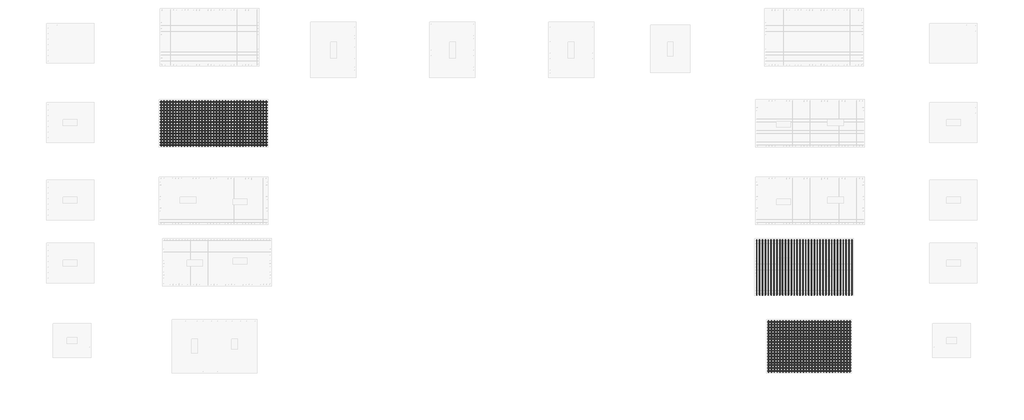
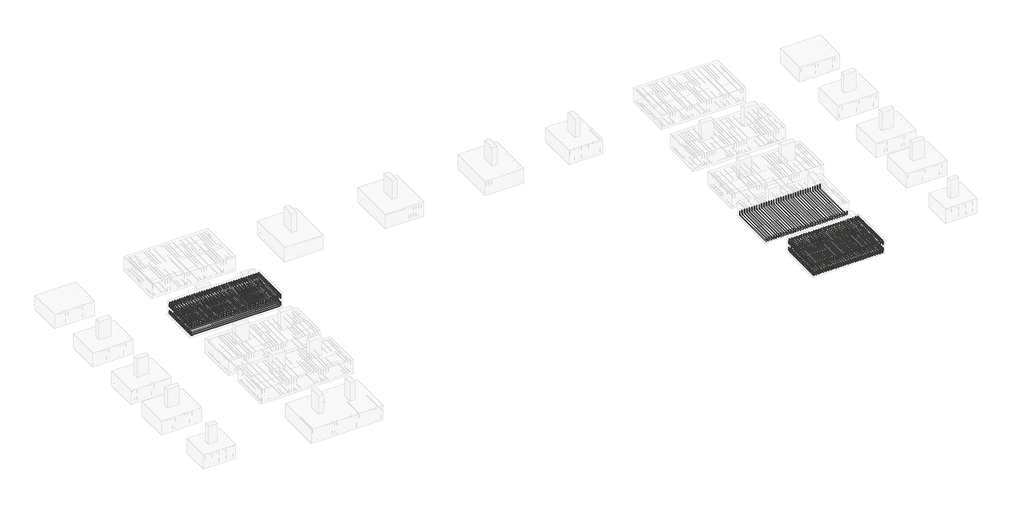
# One storey, part 6 of 21: 8 reinforcing bars.
"""IFC4 building model written with IfcOpenShell, lengths in millimetres."""

from ifc_helpers import new_model, si_unit, point, frame, origin, place, context, project, spatial, polyline, circle_curve, trimmed, segment, composite_curve, source, transform, mapped, element, save
from ifc_brep_helpers import swept_disk

model = new_model("IFC4")

# Units and contexts
model_context = context("Model", 3, world=origin())
ifc_project = project(units=[si_unit("LENGTHUNIT", "METRE", prefix="MILLI")], contexts=[model_context])

# Site, building, storey
site = spatial("IfcSite", under=ifc_project)
building = spatial("IfcBuilding", under=site)
storey = spatial("IfcBuildingStorey", under=building, Elevation=-1100.0)

# Reinforcing bars
placement = place(None, origin())
reinforcing_bar_shape = source(origin(), model_context, "Body", "SolidModel", [
    swept_disk(composite_curve([segment(polyline([(-19614.5839151, -1642.8795712, -1400.0), (-19614.5839151, -1642.8795712, -1213.4)]), True, "CONTINUOUS"), segment(trimmed(circle_curve(frame((-19614.5839151, -1587.4295712, -1213.4), z_axis=(-1.0, 0.0, 0.0), x_axis=(0.0, -55.450000000000045, 0.0)), 55.45), [point((-19614.5839151, -1642.8795712, -1213.4))], [point((-19614.5839151, -1587.4295712, -1157.95))], True, "CARTESIAN"), True, "CONTINUOUS"), segment(polyline([(-19614.5839151, -1587.4295712, -1157.95), (-19614.5839151, 585.7704288, -1157.95)]), True, "CONTINUOUS"), segment(trimmed(circle_curve(frame((-19614.5839151, 585.7704288, -1213.4), z_axis=(-1.0, 0.0, 0.0), x_axis=(0.0, 0.0, 55.450000000000045)), 55.45), [point((-19614.5839151, 585.7704288, -1157.95))], [point((-19614.5839151, 641.2204288, -1213.4))], True, "CARTESIAN"), True, "CONTINUOUS"), segment(polyline([(-19614.5839151, 641.2204288, -1213.4), (-19614.5839151, 641.2204288, -1400.0)]), True, "CONTINUOUS")], self_intersect=False), 7.95),
])
element("IfcReinforcingBar", 1, at=placement, inside=storey, context=model_context, shape_type="MappedRepresentation", body=[
    mapped(reinforcing_bar_shape, transform((0.0, 0.0, 0.0), x_axis=(1.0, 0.0, 0.0), y_axis=(0.0, 1.0, 0.0), z_axis=(0.0, 0.0, 1.0))),
    mapped(reinforcing_bar_shape, transform((147.2696553, 0.0, 0.0), x_axis=(1.0, 0.0, 0.0), y_axis=(0.0, 1.0, 0.0), z_axis=(0.0, 0.0, 1.0))),
    mapped(reinforcing_bar_shape, transform((294.5393106, 0.0, 0.0), x_axis=(1.0, 0.0, 0.0), y_axis=(0.0, 1.0, 0.0), z_axis=(0.0, 0.0, 1.0))),
    mapped(reinforcing_bar_shape, transform((441.8089659, 0.0, 0.0), x_axis=(1.0, 0.0, 0.0), y_axis=(0.0, 1.0, 0.0), z_axis=(0.0, 0.0, 1.0))),
    mapped(reinforcing_bar_shape, transform((589.0786213, 0.0, 0.0), x_axis=(1.0, 0.0, 0.0), y_axis=(0.0, 1.0, 0.0), z_axis=(0.0, 0.0, 1.0))),
    mapped(reinforcing_bar_shape, transform((736.3482766, 0.0, 0.0), x_axis=(1.0, 0.0, 0.0), y_axis=(0.0, 1.0, 0.0), z_axis=(0.0, 0.0, 1.0))),
    mapped(reinforcing_bar_shape, transform((883.6179319, 0.0, 0.0), x_axis=(1.0, 0.0, 0.0), y_axis=(0.0, 1.0, 0.0), z_axis=(0.0, 0.0, 1.0))),
    mapped(reinforcing_bar_shape, transform((1030.8875872, 0.0, 0.0), x_axis=(1.0, 0.0, 0.0), y_axis=(0.0, 1.0, 0.0), z_axis=(0.0, 0.0, 1.0))),
    mapped(reinforcing_bar_shape, transform((1178.1572425, 0.0, 0.0), x_axis=(1.0, 0.0, 0.0), y_axis=(0.0, 1.0, 0.0), z_axis=(0.0, 0.0, 1.0))),
    mapped(reinforcing_bar_shape, transform((1325.4268978, 0.0, 0.0), x_axis=(1.0, 0.0, 0.0), y_axis=(0.0, 1.0, 0.0), z_axis=(0.0, 0.0, 1.0))),
    mapped(reinforcing_bar_shape, transform((1472.6965532, 0.0, 0.0), x_axis=(1.0, 0.0, 0.0), y_axis=(0.0, 1.0, 0.0), z_axis=(0.0, 0.0, 1.0))),
    mapped(reinforcing_bar_shape, transform((1619.9662085, 0.0, 0.0), x_axis=(1.0, 0.0, 0.0), y_axis=(0.0, 1.0, 0.0), z_axis=(0.0, 0.0, 1.0))),
    mapped(reinforcing_bar_shape, transform((1767.2358638, 0.0, 0.0), x_axis=(1.0, 0.0, 0.0), y_axis=(0.0, 1.0, 0.0), z_axis=(0.0, 0.0, 1.0))),
    mapped(reinforcing_bar_shape, transform((1914.5055191, 0.0, 0.0), x_axis=(1.0, 0.0, 0.0), y_axis=(0.0, 1.0, 0.0), z_axis=(0.0, 0.0, 1.0))),
    mapped(reinforcing_bar_shape, transform((2061.7751744, 0.0, 0.0), x_axis=(1.0, 0.0, 0.0), y_axis=(0.0, 1.0, 0.0), z_axis=(0.0, 0.0, 1.0))),
    mapped(reinforcing_bar_shape, transform((2209.0448297, 0.0, 0.0), x_axis=(1.0, 0.0, 0.0), y_axis=(0.0, 1.0, 0.0), z_axis=(0.0, 0.0, 1.0))),
    mapped(reinforcing_bar_shape, transform((2356.314485, 0.0, 0.0), x_axis=(1.0, 0.0, 0.0), y_axis=(0.0, 1.0, 0.0), z_axis=(0.0, 0.0, 1.0))),
    mapped(reinforcing_bar_shape, transform((2503.5841404, 0.0, 0.0), x_axis=(1.0, 0.0, 0.0), y_axis=(0.0, 1.0, 0.0), z_axis=(0.0, 0.0, 1.0))),
    mapped(reinforcing_bar_shape, transform((2650.8537957, 0.0, 0.0), x_axis=(1.0, 0.0, 0.0), y_axis=(0.0, 1.0, 0.0), z_axis=(0.0, 0.0, 1.0))),
    mapped(reinforcing_bar_shape, transform((2798.123451, 0.0, 0.0), x_axis=(1.0, 0.0, 0.0), y_axis=(0.0, 1.0, 0.0), z_axis=(0.0, 0.0, 1.0))),
    mapped(reinforcing_bar_shape, transform((2945.3931063, 0.0, 0.0), x_axis=(1.0, 0.0, 0.0), y_axis=(0.0, 1.0, 0.0), z_axis=(0.0, 0.0, 1.0))),
    mapped(reinforcing_bar_shape, transform((3092.6627616, 0.0, 0.0), x_axis=(1.0, 0.0, 0.0), y_axis=(0.0, 1.0, 0.0), z_axis=(0.0, 0.0, 1.0))),
    mapped(reinforcing_bar_shape, transform((3239.9324169, 0.0, 0.0), x_axis=(1.0, 0.0, 0.0), y_axis=(0.0, 1.0, 0.0), z_axis=(0.0, 0.0, 1.0))),
    mapped(reinforcing_bar_shape, transform((3387.2020722, 0.0, 0.0), x_axis=(1.0, 0.0, 0.0), y_axis=(0.0, 1.0, 0.0), z_axis=(0.0, 0.0, 1.0))),
    mapped(reinforcing_bar_shape, transform((3534.4717276, 0.0, 0.0), x_axis=(1.0, 0.0, 0.0), y_axis=(0.0, 1.0, 0.0), z_axis=(0.0, 0.0, 1.0))),
    mapped(reinforcing_bar_shape, transform((3681.7413829, 0.0, 0.0), x_axis=(1.0, 0.0, 0.0), y_axis=(0.0, 1.0, 0.0), z_axis=(0.0, 0.0, 1.0))),
    mapped(reinforcing_bar_shape, transform((3829.0110382, 0.0, 0.0), x_axis=(1.0, 0.0, 0.0), y_axis=(0.0, 1.0, 0.0), z_axis=(0.0, 0.0, 1.0))),
    mapped(reinforcing_bar_shape, transform((3976.2806935, 0.0, 0.0), x_axis=(1.0, 0.0, 0.0), y_axis=(0.0, 1.0, 0.0), z_axis=(0.0, 0.0, 1.0))),
    mapped(reinforcing_bar_shape, transform((4123.5503488, 0.0, 0.0), x_axis=(1.0, 0.0, 0.0), y_axis=(0.0, 1.0, 0.0), z_axis=(0.0, 0.0, 1.0))),
    mapped(reinforcing_bar_shape, transform((4270.8200041, 0.0, 0.0), x_axis=(1.0, 0.0, 0.0), y_axis=(0.0, 1.0, 0.0), z_axis=(0.0, 0.0, 1.0))),
    mapped(reinforcing_bar_shape, transform((4418.0896595, 0.0, 0.0), x_axis=(1.0, 0.0, 0.0), y_axis=(0.0, 1.0, 0.0), z_axis=(0.0, 0.0, 1.0))),
    mapped(reinforcing_bar_shape, transform((4565.3593148, 0.0, 0.0), x_axis=(1.0, 0.0, 0.0), y_axis=(0.0, 1.0, 0.0), z_axis=(0.0, 0.0, 1.0))),
    mapped(reinforcing_bar_shape, transform((4712.6289701, 0.0, 0.0), x_axis=(1.0, 0.0, 0.0), y_axis=(0.0, 1.0, 0.0), z_axis=(0.0, 0.0, 1.0))),
    mapped(reinforcing_bar_shape, transform((4859.8986254, 0.0, 0.0), x_axis=(1.0, 0.0, 0.0), y_axis=(0.0, 1.0, 0.0), z_axis=(0.0, 0.0, 1.0))),
    mapped(reinforcing_bar_shape, transform((5007.1682807, 0.0, 0.0), x_axis=(1.0, 0.0, 0.0), y_axis=(0.0, 1.0, 0.0), z_axis=(0.0, 0.0, 1.0))),
    mapped(reinforcing_bar_shape, transform((5154.437936, 0.0, 0.0), x_axis=(1.0, 0.0, 0.0), y_axis=(0.0, 1.0, 0.0), z_axis=(0.0, 0.0, 1.0))),
    mapped(reinforcing_bar_shape, transform((5301.7075913, 0.0, 0.0), x_axis=(1.0, 0.0, 0.0), y_axis=(0.0, 1.0, 0.0), z_axis=(0.0, 0.0, 1.0))),
])
reinforcing_bar_2_shape = source(origin(), model_context, "Body", "SolidModel", [
    swept_disk(composite_curve([segment(polyline([(-19652.8826863, 589.3862648, -1428.1111113), (-19652.8826863, 589.3862648, -1241.5111113)]), True, "CONTINUOUS"), segment(trimmed(circle_curve(frame((-19597.4326863, 589.3862648, -1241.5111113), z_axis=(0.0, 1.0, 0.0), x_axis=(-55.45000000000073, 0.0, 0.0)), 55.45), [point((-19652.8826863, 589.3862648, -1241.5111113))], [point((-19597.4326863, 589.3862648, -1186.0611113))], True, "CARTESIAN"), True, "CONTINUOUS"), segment(polyline([(-19597.4326863, 589.3862648, -1186.0611113), (-14324.2326863, 589.3862648, -1186.0611113)]), True, "CONTINUOUS"), segment(trimmed(circle_curve(frame((-14324.2326863, 589.3862648, -1241.5111113), z_axis=(0.0, 1.0, 0.0), x_axis=(0.0, 0.0, 55.450000000000045)), 55.45), [point((-14324.2326863, 589.3862648, -1186.0611113))], [point((-14268.7826863, 589.3862648, -1241.5111113))], True, "CARTESIAN"), True, "CONTINUOUS"), segment(polyline([(-14268.7826863, 589.3862648, -1241.5111113), (-14268.7826863, 589.3862648, -1428.1111113)]), True, "CONTINUOUS")], self_intersect=False), 7.95),
])
element("IfcReinforcingBar", 2, at=placement, inside=storey, context=model_context, shape_type="MappedRepresentation", body=[
    mapped(reinforcing_bar_2_shape, transform((0.0, 0.0, 0.0), x_axis=(1.0, 0.0, 0.0), y_axis=(0.0, 1.0, 0.0), z_axis=(0.0, 0.0, 1.0))),
    mapped(reinforcing_bar_2_shape, transform((0.0, -145.2528929, 0.0), x_axis=(1.0, 0.0, 0.0), y_axis=(0.0, 1.0, 0.0), z_axis=(0.0, 0.0, 1.0))),
    mapped(reinforcing_bar_2_shape, transform((0.0, -290.5057858, 0.0), x_axis=(1.0, 0.0, 0.0), y_axis=(0.0, 1.0, 0.0), z_axis=(0.0, 0.0, 1.0))),
    mapped(reinforcing_bar_2_shape, transform((0.0, -435.7586787, 0.0), x_axis=(1.0, 0.0, 0.0), y_axis=(0.0, 1.0, 0.0), z_axis=(0.0, 0.0, 1.0))),
    mapped(reinforcing_bar_2_shape, transform((0.0, -581.0115716, 0.0), x_axis=(1.0, 0.0, 0.0), y_axis=(0.0, 1.0, 0.0), z_axis=(0.0, 0.0, 1.0))),
    mapped(reinforcing_bar_2_shape, transform((0.0, -726.2644645, 0.0), x_axis=(1.0, 0.0, 0.0), y_axis=(0.0, 1.0, 0.0), z_axis=(0.0, 0.0, 1.0))),
    mapped(reinforcing_bar_2_shape, transform((0.0, -871.5173574, 0.0), x_axis=(1.0, 0.0, 0.0), y_axis=(0.0, 1.0, 0.0), z_axis=(0.0, 0.0, 1.0))),
    mapped(reinforcing_bar_2_shape, transform((0.0, -1016.7702503, 0.0), x_axis=(1.0, 0.0, 0.0), y_axis=(0.0, 1.0, 0.0), z_axis=(0.0, 0.0, 1.0))),
    mapped(reinforcing_bar_2_shape, transform((0.0, -1162.0231432, 0.0), x_axis=(1.0, 0.0, 0.0), y_axis=(0.0, 1.0, 0.0), z_axis=(0.0, 0.0, 1.0))),
    mapped(reinforcing_bar_2_shape, transform((0.0, -1307.276036, 0.0), x_axis=(1.0, 0.0, 0.0), y_axis=(0.0, 1.0, 0.0), z_axis=(0.0, 0.0, 1.0))),
    mapped(reinforcing_bar_2_shape, transform((0.0, -1452.5289289, 0.0), x_axis=(1.0, 0.0, 0.0), y_axis=(0.0, 1.0, 0.0), z_axis=(0.0, 0.0, 1.0))),
    mapped(reinforcing_bar_2_shape, transform((0.0, -1597.7818218, 0.0), x_axis=(1.0, 0.0, 0.0), y_axis=(0.0, 1.0, 0.0), z_axis=(0.0, 0.0, 1.0))),
    mapped(reinforcing_bar_2_shape, transform((0.0, -1743.0347147, 0.0), x_axis=(1.0, 0.0, 0.0), y_axis=(0.0, 1.0, 0.0), z_axis=(0.0, 0.0, 1.0))),
    mapped(reinforcing_bar_2_shape, transform((0.0, -1888.2876076, 0.0), x_axis=(1.0, 0.0, 0.0), y_axis=(0.0, 1.0, 0.0), z_axis=(0.0, 0.0, 1.0))),
    mapped(reinforcing_bar_2_shape, transform((0.0, -2033.5405005, 0.0), x_axis=(1.0, 0.0, 0.0), y_axis=(0.0, 1.0, 0.0), z_axis=(0.0, 0.0, 1.0))),
    mapped(reinforcing_bar_2_shape, transform((0.0, -2178.7933934, 0.0), x_axis=(1.0, 0.0, 0.0), y_axis=(0.0, 1.0, 0.0), z_axis=(0.0, 0.0, 1.0))),
])
reinforcing_bar_3_shape = source(origin(), model_context, "Body", "SolidModel", [
    swept_disk(composite_curve([segment(polyline([(-19650.8326863, -1589.4071286, -1669.8442859), (-19650.8326863, -1589.4071286, -1852.3442859)]), True, "CONTINUOUS"), segment(trimmed(circle_curve(frame((-19593.3326863, -1589.4071286, -1852.3442859), z_axis=(0.0, -1.0, 0.0), x_axis=(-57.5, 0.0, 0.0)), 57.5), [point((-19650.8326863, -1589.4071286, -1852.3442859))], [point((-19593.3326863, -1589.4071286, -1909.8442859))], True, "CARTESIAN"), True, "CONTINUOUS"), segment(polyline([(-19593.3326863, -1589.4071286, -1909.8442859), (-14328.3326863, -1589.4071286, -1909.8442859)]), True, "CONTINUOUS"), segment(trimmed(circle_curve(frame((-14328.3326863, -1589.4071286, -1852.3442859), z_axis=(0.0, -1.0, 0.0), x_axis=(0.0, 0.0, -57.5)), 57.5), [point((-14328.3326863, -1589.4071286, -1909.8442859))], [point((-14270.8326863, -1589.4071286, -1852.3442859))], True, "CARTESIAN"), True, "CONTINUOUS"), segment(polyline([(-14270.8326863, -1589.4071286, -1852.3442859), (-14270.8326863, -1589.4071286, -1669.8442859)]), True, "CONTINUOUS")], self_intersect=False), 10.0),
])
element("IfcReinforcingBar", 3, at=placement, inside=storey, context=model_context, shape_type="MappedRepresentation", body=[
    mapped(reinforcing_bar_3_shape, transform((0.0, 0.0, 0.0), x_axis=(1.0, 0.0, 0.0), y_axis=(0.0, 1.0, 0.0), z_axis=(0.0, 0.0, 1.0))),
    mapped(reinforcing_bar_3_shape, transform((0.0, 145.2528929, 0.0), x_axis=(1.0, 0.0, 0.0), y_axis=(0.0, 1.0, 0.0), z_axis=(0.0, 0.0, 1.0))),
    mapped(reinforcing_bar_3_shape, transform((0.0, 290.5057858, 0.0), x_axis=(1.0, 0.0, 0.0), y_axis=(0.0, 1.0, 0.0), z_axis=(0.0, 0.0, 1.0))),
    mapped(reinforcing_bar_3_shape, transform((0.0, 435.7586787, 0.0), x_axis=(1.0, 0.0, 0.0), y_axis=(0.0, 1.0, 0.0), z_axis=(0.0, 0.0, 1.0))),
    mapped(reinforcing_bar_3_shape, transform((0.0, 581.0115716, 0.0), x_axis=(1.0, 0.0, 0.0), y_axis=(0.0, 1.0, 0.0), z_axis=(0.0, 0.0, 1.0))),
    mapped(reinforcing_bar_3_shape, transform((0.0, 726.2644645, 0.0), x_axis=(1.0, 0.0, 0.0), y_axis=(0.0, 1.0, 0.0), z_axis=(0.0, 0.0, 1.0))),
    mapped(reinforcing_bar_3_shape, transform((0.0, 871.5173574, 0.0), x_axis=(1.0, 0.0, 0.0), y_axis=(0.0, 1.0, 0.0), z_axis=(0.0, 0.0, 1.0))),
    mapped(reinforcing_bar_3_shape, transform((0.0, 1016.7702503, 0.0), x_axis=(1.0, 0.0, 0.0), y_axis=(0.0, 1.0, 0.0), z_axis=(0.0, 0.0, 1.0))),
    mapped(reinforcing_bar_3_shape, transform((0.0, 1162.0231432, 0.0), x_axis=(1.0, 0.0, 0.0), y_axis=(0.0, 1.0, 0.0), z_axis=(0.0, 0.0, 1.0))),
    mapped(reinforcing_bar_3_shape, transform((0.0, 1307.276036, 0.0), x_axis=(1.0, 0.0, 0.0), y_axis=(0.0, 1.0, 0.0), z_axis=(0.0, 0.0, 1.0))),
    mapped(reinforcing_bar_3_shape, transform((0.0, 1452.5289289, 0.0), x_axis=(1.0, 0.0, 0.0), y_axis=(0.0, 1.0, 0.0), z_axis=(0.0, 0.0, 1.0))),
    mapped(reinforcing_bar_3_shape, transform((0.0, 1597.7818218, 0.0), x_axis=(1.0, 0.0, 0.0), y_axis=(0.0, 1.0, 0.0), z_axis=(0.0, 0.0, 1.0))),
    mapped(reinforcing_bar_3_shape, transform((0.0, 1743.0347147, 0.0), x_axis=(1.0, 0.0, 0.0), y_axis=(0.0, 1.0, 0.0), z_axis=(0.0, 0.0, 1.0))),
    mapped(reinforcing_bar_3_shape, transform((0.0, 1888.2876076, 0.0), x_axis=(1.0, 0.0, 0.0), y_axis=(0.0, 1.0, 0.0), z_axis=(0.0, 0.0, 1.0))),
    mapped(reinforcing_bar_3_shape, transform((0.0, 2033.5405005, 0.0), x_axis=(1.0, 0.0, 0.0), y_axis=(0.0, 1.0, 0.0), z_axis=(0.0, 0.0, 1.0))),
    mapped(reinforcing_bar_3_shape, transform((0.0, 2178.7933934, 0.0), x_axis=(1.0, 0.0, 0.0), y_axis=(0.0, 1.0, 0.0), z_axis=(0.0, 0.0, 1.0))),
])
reinforcing_bar_4_shape = source(origin(), model_context, "Body", "SolidModel", [
    swept_disk(composite_curve([segment(polyline([(10440.4160849, -6360.8295712, -1700.0), (10440.4160849, -6360.8295712, -1882.5)]), True, "CONTINUOUS"), segment(trimmed(circle_curve(frame((10440.4160849, -6418.3295712, -1882.5), z_axis=(-1.0, 0.0, 0.0), x_axis=(0.0, 57.5, 0.0)), 57.5), [point((10440.4160849, -6360.8295712, -1882.5))], [point((10440.4160849, -6418.3295712, -1940.0))], True, "CARTESIAN"), True, "CONTINUOUS"), segment(polyline([(10440.4160849, -6418.3295712, -1940.0), (10440.4160849, -9083.3295712, -1940.0)]), True, "CONTINUOUS"), segment(trimmed(circle_curve(frame((10440.4160849, -9083.3295712, -1882.5), z_axis=(-1.0, 0.0, 0.0), x_axis=(0.0, 0.0, -57.5)), 57.5), [point((10440.4160849, -9083.3295712, -1940.0))], [point((10440.4160849, -9140.8295712, -1882.5))], True, "CARTESIAN"), True, "CONTINUOUS"), segment(polyline([(10440.4160849, -9140.8295712, -1882.5), (10440.4160849, -9140.8295712, -1700.0)]), True, "CONTINUOUS")], self_intersect=False), 10.0),
])
element("IfcReinforcingBar", 4, at=placement, inside=storey, context=model_context, shape_type="MappedRepresentation", body=[
    mapped(reinforcing_bar_4_shape, transform((0.0, 0.0, 0.0), x_axis=(1.0, 0.0, 0.0), y_axis=(0.0, 1.0, 0.0), z_axis=(0.0, 0.0, 1.0))),
    mapped(reinforcing_bar_4_shape, transform((145.5062906, 0.0, 0.0), x_axis=(1.0, 0.0, 0.0), y_axis=(0.0, 1.0, 0.0), z_axis=(0.0, 0.0, 1.0))),
    mapped(reinforcing_bar_4_shape, transform((291.0125813, 0.0, 0.0), x_axis=(1.0, 0.0, 0.0), y_axis=(0.0, 1.0, 0.0), z_axis=(0.0, 0.0, 1.0))),
    mapped(reinforcing_bar_4_shape, transform((436.5188719, 0.0, 0.0), x_axis=(1.0, 0.0, 0.0), y_axis=(0.0, 1.0, 0.0), z_axis=(0.0, 0.0, 1.0))),
    mapped(reinforcing_bar_4_shape, transform((582.0251626, 0.0, 0.0), x_axis=(1.0, 0.0, 0.0), y_axis=(0.0, 1.0, 0.0), z_axis=(0.0, 0.0, 1.0))),
    mapped(reinforcing_bar_4_shape, transform((727.5314532, 0.0, 0.0), x_axis=(1.0, 0.0, 0.0), y_axis=(0.0, 1.0, 0.0), z_axis=(0.0, 0.0, 1.0))),
    mapped(reinforcing_bar_4_shape, transform((873.0377439, 0.0, 0.0), x_axis=(1.0, 0.0, 0.0), y_axis=(0.0, 1.0, 0.0), z_axis=(0.0, 0.0, 1.0))),
    mapped(reinforcing_bar_4_shape, transform((1018.5440345, 0.0, 0.0), x_axis=(1.0, 0.0, 0.0), y_axis=(0.0, 1.0, 0.0), z_axis=(0.0, 0.0, 1.0))),
    mapped(reinforcing_bar_4_shape, transform((1164.0503252, 0.0, 0.0), x_axis=(1.0, 0.0, 0.0), y_axis=(0.0, 1.0, 0.0), z_axis=(0.0, 0.0, 1.0))),
    mapped(reinforcing_bar_4_shape, transform((1309.5566158, 0.0, 0.0), x_axis=(1.0, 0.0, 0.0), y_axis=(0.0, 1.0, 0.0), z_axis=(0.0, 0.0, 1.0))),
    mapped(reinforcing_bar_4_shape, transform((1455.0629065, 0.0, 0.0), x_axis=(1.0, 0.0, 0.0), y_axis=(0.0, 1.0, 0.0), z_axis=(0.0, 0.0, 1.0))),
    mapped(reinforcing_bar_4_shape, transform((1600.5691971, 0.0, 0.0), x_axis=(1.0, 0.0, 0.0), y_axis=(0.0, 1.0, 0.0), z_axis=(0.0, 0.0, 1.0))),
    mapped(reinforcing_bar_4_shape, transform((1746.0754878, 0.0, 0.0), x_axis=(1.0, 0.0, 0.0), y_axis=(0.0, 1.0, 0.0), z_axis=(0.0, 0.0, 1.0))),
    mapped(reinforcing_bar_4_shape, transform((1891.5817784, 0.0, 0.0), x_axis=(1.0, 0.0, 0.0), y_axis=(0.0, 1.0, 0.0), z_axis=(0.0, 0.0, 1.0))),
    mapped(reinforcing_bar_4_shape, transform((2037.0880691, 0.0, 0.0), x_axis=(1.0, 0.0, 0.0), y_axis=(0.0, 1.0, 0.0), z_axis=(0.0, 0.0, 1.0))),
    mapped(reinforcing_bar_4_shape, transform((2182.5943597, 0.0, 0.0), x_axis=(1.0, 0.0, 0.0), y_axis=(0.0, 1.0, 0.0), z_axis=(0.0, 0.0, 1.0))),
    mapped(reinforcing_bar_4_shape, transform((2328.1006504, 0.0, 0.0), x_axis=(1.0, 0.0, 0.0), y_axis=(0.0, 1.0, 0.0), z_axis=(0.0, 0.0, 1.0))),
    mapped(reinforcing_bar_4_shape, transform((2473.606941, 0.0, 0.0), x_axis=(1.0, 0.0, 0.0), y_axis=(0.0, 1.0, 0.0), z_axis=(0.0, 0.0, 1.0))),
    mapped(reinforcing_bar_4_shape, transform((2619.1132316, 0.0, 0.0), x_axis=(1.0, 0.0, 0.0), y_axis=(0.0, 1.0, 0.0), z_axis=(0.0, 0.0, 1.0))),
    mapped(reinforcing_bar_4_shape, transform((2764.6195223, 0.0, 0.0), x_axis=(1.0, 0.0, 0.0), y_axis=(0.0, 1.0, 0.0), z_axis=(0.0, 0.0, 1.0))),
    mapped(reinforcing_bar_4_shape, transform((2910.1258129, 0.0, 0.0), x_axis=(1.0, 0.0, 0.0), y_axis=(0.0, 1.0, 0.0), z_axis=(0.0, 0.0, 1.0))),
    mapped(reinforcing_bar_4_shape, transform((3055.6321036, 0.0, 0.0), x_axis=(1.0, 0.0, 0.0), y_axis=(0.0, 1.0, 0.0), z_axis=(0.0, 0.0, 1.0))),
    mapped(reinforcing_bar_4_shape, transform((3201.1383942, 0.0, 0.0), x_axis=(1.0, 0.0, 0.0), y_axis=(0.0, 1.0, 0.0), z_axis=(0.0, 0.0, 1.0))),
    mapped(reinforcing_bar_4_shape, transform((3346.6446849, 0.0, 0.0), x_axis=(1.0, 0.0, 0.0), y_axis=(0.0, 1.0, 0.0), z_axis=(0.0, 0.0, 1.0))),
    mapped(reinforcing_bar_4_shape, transform((3492.1509755, 0.0, 0.0), x_axis=(1.0, 0.0, 0.0), y_axis=(0.0, 1.0, 0.0), z_axis=(0.0, 0.0, 1.0))),
    mapped(reinforcing_bar_4_shape, transform((3637.6572662, 0.0, 0.0), x_axis=(1.0, 0.0, 0.0), y_axis=(0.0, 1.0, 0.0), z_axis=(0.0, 0.0, 1.0))),
    mapped(reinforcing_bar_4_shape, transform((3783.1635568, 0.0, 0.0), x_axis=(1.0, 0.0, 0.0), y_axis=(0.0, 1.0, 0.0), z_axis=(0.0, 0.0, 1.0))),
    mapped(reinforcing_bar_4_shape, transform((3928.6698475, 0.0, 0.0), x_axis=(1.0, 0.0, 0.0), y_axis=(0.0, 1.0, 0.0), z_axis=(0.0, 0.0, 1.0))),
    mapped(reinforcing_bar_4_shape, transform((4074.1761381, 0.0, 0.0), x_axis=(1.0, 0.0, 0.0), y_axis=(0.0, 1.0, 0.0), z_axis=(0.0, 0.0, 1.0))),
    mapped(reinforcing_bar_4_shape, transform((4219.6824288, 0.0, 0.0), x_axis=(1.0, 0.0, 0.0), y_axis=(0.0, 1.0, 0.0), z_axis=(0.0, 0.0, 1.0))),
    mapped(reinforcing_bar_4_shape, transform((4365.1887194, 0.0, 0.0), x_axis=(1.0, 0.0, 0.0), y_axis=(0.0, 1.0, 0.0), z_axis=(0.0, 0.0, 1.0))),
    mapped(reinforcing_bar_4_shape, transform((4510.6950101, 0.0, 0.0), x_axis=(1.0, 0.0, 0.0), y_axis=(0.0, 1.0, 0.0), z_axis=(0.0, 0.0, 1.0))),
    mapped(reinforcing_bar_4_shape, transform((4656.2013007, 0.0, 0.0), x_axis=(1.0, 0.0, 0.0), y_axis=(0.0, 1.0, 0.0), z_axis=(0.0, 0.0, 1.0))),
    mapped(reinforcing_bar_4_shape, transform((4801.7075913, 0.0, 0.0), x_axis=(1.0, 0.0, 0.0), y_axis=(0.0, 1.0, 0.0), z_axis=(0.0, 0.0, 1.0))),
])
reinforcing_bar_5_shape = source(origin(), model_context, "Body", "SolidModel", [
    swept_disk(composite_curve([segment(polyline([(11035.4160849, -10455.8295712, -1700.0), (11035.4160849, -10455.8295712, -1882.5)]), True, "CONTINUOUS"), segment(trimmed(circle_curve(frame((11035.4160849, -10513.3295712, -1882.5), z_axis=(-1.0, 0.0, 0.0), x_axis=(0.0, 57.5, 0.0)), 57.5), [point((11035.4160849, -10455.8295712, -1882.5))], [point((11035.4160849, -10513.3295712, -1940.0))], True, "CARTESIAN"), True, "CONTINUOUS"), segment(polyline([(11035.4160849, -10513.3295712, -1940.0), (11035.4160849, -12978.3295712, -1940.0)]), True, "CONTINUOUS"), segment(trimmed(circle_curve(frame((11035.4160849, -12978.3295712, -1882.5), z_axis=(-1.0, 0.0, 0.0), x_axis=(0.0, 0.0, -57.5)), 57.5), [point((11035.4160849, -12978.3295712, -1940.0))], [point((11035.4160849, -13035.8295712, -1882.5))], True, "CARTESIAN"), True, "CONTINUOUS"), segment(polyline([(11035.4160849, -13035.8295712, -1882.5), (11035.4160849, -13035.8295712, -1700.0)]), True, "CONTINUOUS")], self_intersect=False), 10.0),
])
element("IfcReinforcingBar", 5, at=placement, inside=storey, context=model_context, shape_type="MappedRepresentation", body=[
    mapped(reinforcing_bar_5_shape, transform((0.0, 0.0, 0.0), x_axis=(1.0, 0.0, 0.0), y_axis=(0.0, 1.0, 0.0), z_axis=(0.0, 0.0, 1.0))),
    mapped(reinforcing_bar_5_shape, transform((146.4895568, 0.0, 0.0), x_axis=(1.0, 0.0, 0.0), y_axis=(0.0, 1.0, 0.0), z_axis=(0.0, 0.0, 1.0))),
    mapped(reinforcing_bar_5_shape, transform((292.9791137, 0.0, 0.0), x_axis=(1.0, 0.0, 0.0), y_axis=(0.0, 1.0, 0.0), z_axis=(0.0, 0.0, 1.0))),
    mapped(reinforcing_bar_5_shape, transform((439.4686705, 0.0, 0.0), x_axis=(1.0, 0.0, 0.0), y_axis=(0.0, 1.0, 0.0), z_axis=(0.0, 0.0, 1.0))),
    mapped(reinforcing_bar_5_shape, transform((585.9582273, 0.0, 0.0), x_axis=(1.0, 0.0, 0.0), y_axis=(0.0, 1.0, 0.0), z_axis=(0.0, 0.0, 1.0))),
    mapped(reinforcing_bar_5_shape, transform((732.4477842, 0.0, 0.0), x_axis=(1.0, 0.0, 0.0), y_axis=(0.0, 1.0, 0.0), z_axis=(0.0, 0.0, 1.0))),
    mapped(reinforcing_bar_5_shape, transform((878.937341, 0.0, 0.0), x_axis=(1.0, 0.0, 0.0), y_axis=(0.0, 1.0, 0.0), z_axis=(0.0, 0.0, 1.0))),
    mapped(reinforcing_bar_5_shape, transform((1025.4268978, 0.0, 0.0), x_axis=(1.0, 0.0, 0.0), y_axis=(0.0, 1.0, 0.0), z_axis=(0.0, 0.0, 1.0))),
    mapped(reinforcing_bar_5_shape, transform((1171.9164547, 0.0, 0.0), x_axis=(1.0, 0.0, 0.0), y_axis=(0.0, 1.0, 0.0), z_axis=(0.0, 0.0, 1.0))),
    mapped(reinforcing_bar_5_shape, transform((1318.4060115, 0.0, 0.0), x_axis=(1.0, 0.0, 0.0), y_axis=(0.0, 1.0, 0.0), z_axis=(0.0, 0.0, 1.0))),
    mapped(reinforcing_bar_5_shape, transform((1464.8955683, 0.0, 0.0), x_axis=(1.0, 0.0, 0.0), y_axis=(0.0, 1.0, 0.0), z_axis=(0.0, 0.0, 1.0))),
    mapped(reinforcing_bar_5_shape, transform((1611.3851252, 0.0, 0.0), x_axis=(1.0, 0.0, 0.0), y_axis=(0.0, 1.0, 0.0), z_axis=(0.0, 0.0, 1.0))),
    mapped(reinforcing_bar_5_shape, transform((1757.874682, 0.0, 0.0), x_axis=(1.0, 0.0, 0.0), y_axis=(0.0, 1.0, 0.0), z_axis=(0.0, 0.0, 1.0))),
    mapped(reinforcing_bar_5_shape, transform((1904.3642388, 0.0, 0.0), x_axis=(1.0, 0.0, 0.0), y_axis=(0.0, 1.0, 0.0), z_axis=(0.0, 0.0, 1.0))),
    mapped(reinforcing_bar_5_shape, transform((2050.8537957, 0.0, 0.0), x_axis=(1.0, 0.0, 0.0), y_axis=(0.0, 1.0, 0.0), z_axis=(0.0, 0.0, 1.0))),
    mapped(reinforcing_bar_5_shape, transform((2197.3433525, 0.0, 0.0), x_axis=(1.0, 0.0, 0.0), y_axis=(0.0, 1.0, 0.0), z_axis=(0.0, 0.0, 1.0))),
    mapped(reinforcing_bar_5_shape, transform((2343.8329093, 0.0, 0.0), x_axis=(1.0, 0.0, 0.0), y_axis=(0.0, 1.0, 0.0), z_axis=(0.0, 0.0, 1.0))),
    mapped(reinforcing_bar_5_shape, transform((2490.3224662, 0.0, 0.0), x_axis=(1.0, 0.0, 0.0), y_axis=(0.0, 1.0, 0.0), z_axis=(0.0, 0.0, 1.0))),
    mapped(reinforcing_bar_5_shape, transform((2636.812023, 0.0, 0.0), x_axis=(1.0, 0.0, 0.0), y_axis=(0.0, 1.0, 0.0), z_axis=(0.0, 0.0, 1.0))),
    mapped(reinforcing_bar_5_shape, transform((2783.3015798, 0.0, 0.0), x_axis=(1.0, 0.0, 0.0), y_axis=(0.0, 1.0, 0.0), z_axis=(0.0, 0.0, 1.0))),
    mapped(reinforcing_bar_5_shape, transform((2929.7911367, 0.0, 0.0), x_axis=(1.0, 0.0, 0.0), y_axis=(0.0, 1.0, 0.0), z_axis=(0.0, 0.0, 1.0))),
    mapped(reinforcing_bar_5_shape, transform((3076.2806935, 0.0, 0.0), x_axis=(1.0, 0.0, 0.0), y_axis=(0.0, 1.0, 0.0), z_axis=(0.0, 0.0, 1.0))),
    mapped(reinforcing_bar_5_shape, transform((3222.7702503, 0.0, 0.0), x_axis=(1.0, 0.0, 0.0), y_axis=(0.0, 1.0, 0.0), z_axis=(0.0, 0.0, 1.0))),
    mapped(reinforcing_bar_5_shape, transform((3369.2598072, 0.0, 0.0), x_axis=(1.0, 0.0, 0.0), y_axis=(0.0, 1.0, 0.0), z_axis=(0.0, 0.0, 1.0))),
    mapped(reinforcing_bar_5_shape, transform((3515.749364, 0.0, 0.0), x_axis=(1.0, 0.0, 0.0), y_axis=(0.0, 1.0, 0.0), z_axis=(0.0, 0.0, 1.0))),
    mapped(reinforcing_bar_5_shape, transform((3662.2389208, 0.0, 0.0), x_axis=(1.0, 0.0, 0.0), y_axis=(0.0, 1.0, 0.0), z_axis=(0.0, 0.0, 1.0))),
    mapped(reinforcing_bar_5_shape, transform((3808.7284777, 0.0, 0.0), x_axis=(1.0, 0.0, 0.0), y_axis=(0.0, 1.0, 0.0), z_axis=(0.0, 0.0, 1.0))),
    mapped(reinforcing_bar_5_shape, transform((3955.2180345, 0.0, 0.0), x_axis=(1.0, 0.0, 0.0), y_axis=(0.0, 1.0, 0.0), z_axis=(0.0, 0.0, 1.0))),
    mapped(reinforcing_bar_5_shape, transform((4101.7075913, 0.0, 0.0), x_axis=(1.0, 0.0, 0.0), y_axis=(0.0, 1.0, 0.0), z_axis=(0.0, 0.0, 1.0))),
])
reinforcing_bar_6_shape = source(origin(), model_context, "Body", "SolidModel", [
    swept_disk(composite_curve([segment(polyline([(11035.4160849, -13037.8795712, -1400.0), (11035.4160849, -13037.8795712, -1213.4)]), True, "CONTINUOUS"), segment(trimmed(circle_curve(frame((11035.4160849, -12982.4295712, -1213.4), z_axis=(-1.0, 0.0, 0.0), x_axis=(0.0, -55.44999999999891, 0.0)), 55.45), [point((11035.4160849, -13037.8795712, -1213.4))], [point((11035.4160849, -12982.4295712, -1157.95))], True, "CARTESIAN"), True, "CONTINUOUS"), segment(polyline([(11035.4160849, -12982.4295712, -1157.95), (11035.4160849, -10509.2295712, -1157.95)]), True, "CONTINUOUS"), segment(trimmed(circle_curve(frame((11035.4160849, -10509.2295712, -1213.4), z_axis=(-1.0, 0.0, 0.0), x_axis=(0.0, 0.0, 55.450000000000045)), 55.45), [point((11035.4160849, -10509.2295712, -1157.95))], [point((11035.4160849, -10453.7795712, -1213.4))], True, "CARTESIAN"), True, "CONTINUOUS"), segment(polyline([(11035.4160849, -10453.7795712, -1213.4), (11035.4160849, -10453.7795712, -1400.0)]), True, "CONTINUOUS")], self_intersect=False), 7.95),
])
element("IfcReinforcingBar", 6, at=placement, inside=storey, context=model_context, shape_type="MappedRepresentation", body=[
    mapped(reinforcing_bar_6_shape, transform((0.0, 0.0, 0.0), x_axis=(1.0, 0.0, 0.0), y_axis=(0.0, 1.0, 0.0), z_axis=(0.0, 0.0, 1.0))),
    mapped(reinforcing_bar_6_shape, transform((146.4895568, 0.0, 0.0), x_axis=(1.0, 0.0, 0.0), y_axis=(0.0, 1.0, 0.0), z_axis=(0.0, 0.0, 1.0))),
    mapped(reinforcing_bar_6_shape, transform((292.9791137, 0.0, 0.0), x_axis=(1.0, 0.0, 0.0), y_axis=(0.0, 1.0, 0.0), z_axis=(0.0, 0.0, 1.0))),
    mapped(reinforcing_bar_6_shape, transform((439.4686705, 0.0, 0.0), x_axis=(1.0, 0.0, 0.0), y_axis=(0.0, 1.0, 0.0), z_axis=(0.0, 0.0, 1.0))),
    mapped(reinforcing_bar_6_shape, transform((585.9582273, 0.0, 0.0), x_axis=(1.0, 0.0, 0.0), y_axis=(0.0, 1.0, 0.0), z_axis=(0.0, 0.0, 1.0))),
    mapped(reinforcing_bar_6_shape, transform((732.4477842, 0.0, 0.0), x_axis=(1.0, 0.0, 0.0), y_axis=(0.0, 1.0, 0.0), z_axis=(0.0, 0.0, 1.0))),
    mapped(reinforcing_bar_6_shape, transform((878.937341, 0.0, 0.0), x_axis=(1.0, 0.0, 0.0), y_axis=(0.0, 1.0, 0.0), z_axis=(0.0, 0.0, 1.0))),
    mapped(reinforcing_bar_6_shape, transform((1025.4268978, 0.0, 0.0), x_axis=(1.0, 0.0, 0.0), y_axis=(0.0, 1.0, 0.0), z_axis=(0.0, 0.0, 1.0))),
    mapped(reinforcing_bar_6_shape, transform((1171.9164547, 0.0, 0.0), x_axis=(1.0, 0.0, 0.0), y_axis=(0.0, 1.0, 0.0), z_axis=(0.0, 0.0, 1.0))),
    mapped(reinforcing_bar_6_shape, transform((1318.4060115, 0.0, 0.0), x_axis=(1.0, 0.0, 0.0), y_axis=(0.0, 1.0, 0.0), z_axis=(0.0, 0.0, 1.0))),
    mapped(reinforcing_bar_6_shape, transform((1464.8955683, 0.0, 0.0), x_axis=(1.0, 0.0, 0.0), y_axis=(0.0, 1.0, 0.0), z_axis=(0.0, 0.0, 1.0))),
    mapped(reinforcing_bar_6_shape, transform((1611.3851252, 0.0, 0.0), x_axis=(1.0, 0.0, 0.0), y_axis=(0.0, 1.0, 0.0), z_axis=(0.0, 0.0, 1.0))),
    mapped(reinforcing_bar_6_shape, transform((1757.874682, 0.0, 0.0), x_axis=(1.0, 0.0, 0.0), y_axis=(0.0, 1.0, 0.0), z_axis=(0.0, 0.0, 1.0))),
    mapped(reinforcing_bar_6_shape, transform((1904.3642388, 0.0, 0.0), x_axis=(1.0, 0.0, 0.0), y_axis=(0.0, 1.0, 0.0), z_axis=(0.0, 0.0, 1.0))),
    mapped(reinforcing_bar_6_shape, transform((2050.8537957, 0.0, 0.0), x_axis=(1.0, 0.0, 0.0), y_axis=(0.0, 1.0, 0.0), z_axis=(0.0, 0.0, 1.0))),
    mapped(reinforcing_bar_6_shape, transform((2197.3433525, 0.0, 0.0), x_axis=(1.0, 0.0, 0.0), y_axis=(0.0, 1.0, 0.0), z_axis=(0.0, 0.0, 1.0))),
    mapped(reinforcing_bar_6_shape, transform((2343.8329093, 0.0, 0.0), x_axis=(1.0, 0.0, 0.0), y_axis=(0.0, 1.0, 0.0), z_axis=(0.0, 0.0, 1.0))),
    mapped(reinforcing_bar_6_shape, transform((2490.3224662, 0.0, 0.0), x_axis=(1.0, 0.0, 0.0), y_axis=(0.0, 1.0, 0.0), z_axis=(0.0, 0.0, 1.0))),
    mapped(reinforcing_bar_6_shape, transform((2636.812023, 0.0, 0.0), x_axis=(1.0, 0.0, 0.0), y_axis=(0.0, 1.0, 0.0), z_axis=(0.0, 0.0, 1.0))),
    mapped(reinforcing_bar_6_shape, transform((2783.3015798, 0.0, 0.0), x_axis=(1.0, 0.0, 0.0), y_axis=(0.0, 1.0, 0.0), z_axis=(0.0, 0.0, 1.0))),
    mapped(reinforcing_bar_6_shape, transform((2929.7911367, 0.0, 0.0), x_axis=(1.0, 0.0, 0.0), y_axis=(0.0, 1.0, 0.0), z_axis=(0.0, 0.0, 1.0))),
    mapped(reinforcing_bar_6_shape, transform((3076.2806935, 0.0, 0.0), x_axis=(1.0, 0.0, 0.0), y_axis=(0.0, 1.0, 0.0), z_axis=(0.0, 0.0, 1.0))),
    mapped(reinforcing_bar_6_shape, transform((3222.7702503, 0.0, 0.0), x_axis=(1.0, 0.0, 0.0), y_axis=(0.0, 1.0, 0.0), z_axis=(0.0, 0.0, 1.0))),
    mapped(reinforcing_bar_6_shape, transform((3369.2598072, 0.0, 0.0), x_axis=(1.0, 0.0, 0.0), y_axis=(0.0, 1.0, 0.0), z_axis=(0.0, 0.0, 1.0))),
    mapped(reinforcing_bar_6_shape, transform((3515.749364, 0.0, 0.0), x_axis=(1.0, 0.0, 0.0), y_axis=(0.0, 1.0, 0.0), z_axis=(0.0, 0.0, 1.0))),
    mapped(reinforcing_bar_6_shape, transform((3662.2389208, 0.0, 0.0), x_axis=(1.0, 0.0, 0.0), y_axis=(0.0, 1.0, 0.0), z_axis=(0.0, 0.0, 1.0))),
    mapped(reinforcing_bar_6_shape, transform((3808.7284777, 0.0, 0.0), x_axis=(1.0, 0.0, 0.0), y_axis=(0.0, 1.0, 0.0), z_axis=(0.0, 0.0, 1.0))),
    mapped(reinforcing_bar_6_shape, transform((3955.2180345, 0.0, 0.0), x_axis=(1.0, 0.0, 0.0), y_axis=(0.0, 1.0, 0.0), z_axis=(0.0, 0.0, 1.0))),
    mapped(reinforcing_bar_6_shape, transform((4101.7075913, 0.0, 0.0), x_axis=(1.0, 0.0, 0.0), y_axis=(0.0, 1.0, 0.0), z_axis=(0.0, 0.0, 1.0))),
])
reinforcing_bar_7_shape = source(origin(), model_context, "Body", "SolidModel", [
    swept_disk(composite_curve([segment(polyline([(10997.1173137, -10505.6137352, -1428.1111113), (10997.1173137, -10505.6137352, -1241.5111113)]), True, "CONTINUOUS"), segment(trimmed(circle_curve(frame((11052.5673137, -10505.6137352, -1241.5111113), z_axis=(0.0, 1.0, 0.0), x_axis=(-55.44999999999891, 0.0, 0.0)), 55.45), [point((10997.1173137, -10505.6137352, -1241.5111113))], [point((11052.5673137, -10505.6137352, -1186.0611113))], True, "CARTESIAN"), True, "CONTINUOUS"), segment(polyline([(11052.5673137, -10505.6137352, -1186.0611113), (15125.7673137, -10505.6137352, -1186.0611113)]), True, "CONTINUOUS"), segment(trimmed(circle_curve(frame((15125.7673137, -10505.6137352, -1241.5111113), z_axis=(0.0, 1.0, 0.0), x_axis=(0.0, 0.0, 55.450000000000045)), 55.45), [point((15125.7673137, -10505.6137352, -1186.0611113))], [point((15181.2173137, -10505.6137352, -1241.5111113))], True, "CARTESIAN"), True, "CONTINUOUS"), segment(polyline([(15181.2173137, -10505.6137352, -1241.5111113), (15181.2173137, -10505.6137352, -1428.1111113)]), True, "CONTINUOUS")], self_intersect=False), 7.95),
])
element("IfcReinforcingBar", 7, at=placement, inside=storey, context=model_context, shape_type="MappedRepresentation", body=[
    mapped(reinforcing_bar_7_shape, transform((0.0, 0.0, 0.0), x_axis=(1.0, 0.0, 0.0), y_axis=(0.0, 1.0, 0.0), z_axis=(0.0, 0.0, 1.0))),
    mapped(reinforcing_bar_7_shape, transform((0.0, -145.8113761, 0.0), x_axis=(1.0, 0.0, 0.0), y_axis=(0.0, 1.0, 0.0), z_axis=(0.0, 0.0, 1.0))),
    mapped(reinforcing_bar_7_shape, transform((0.0, -291.6227522, 0.0), x_axis=(1.0, 0.0, 0.0), y_axis=(0.0, 1.0, 0.0), z_axis=(0.0, 0.0, 1.0))),
    mapped(reinforcing_bar_7_shape, transform((0.0, -437.4341282, 0.0), x_axis=(1.0, 0.0, 0.0), y_axis=(0.0, 1.0, 0.0), z_axis=(0.0, 0.0, 1.0))),
    mapped(reinforcing_bar_7_shape, transform((0.0, -583.2455043, 0.0), x_axis=(1.0, 0.0, 0.0), y_axis=(0.0, 1.0, 0.0), z_axis=(0.0, 0.0, 1.0))),
    mapped(reinforcing_bar_7_shape, transform((0.0, -729.0568804, 0.0), x_axis=(1.0, 0.0, 0.0), y_axis=(0.0, 1.0, 0.0), z_axis=(0.0, 0.0, 1.0))),
    mapped(reinforcing_bar_7_shape, transform((0.0, -874.8682565, 0.0), x_axis=(1.0, 0.0, 0.0), y_axis=(0.0, 1.0, 0.0), z_axis=(0.0, 0.0, 1.0))),
    mapped(reinforcing_bar_7_shape, transform((0.0, -1020.6796326, 0.0), x_axis=(1.0, 0.0, 0.0), y_axis=(0.0, 1.0, 0.0), z_axis=(0.0, 0.0, 1.0))),
    mapped(reinforcing_bar_7_shape, transform((0.0, -1166.4910087, 0.0), x_axis=(1.0, 0.0, 0.0), y_axis=(0.0, 1.0, 0.0), z_axis=(0.0, 0.0, 1.0))),
    mapped(reinforcing_bar_7_shape, transform((0.0, -1312.3023847, 0.0), x_axis=(1.0, 0.0, 0.0), y_axis=(0.0, 1.0, 0.0), z_axis=(0.0, 0.0, 1.0))),
    mapped(reinforcing_bar_7_shape, transform((0.0, -1458.1137608, 0.0), x_axis=(1.0, 0.0, 0.0), y_axis=(0.0, 1.0, 0.0), z_axis=(0.0, 0.0, 1.0))),
    mapped(reinforcing_bar_7_shape, transform((0.0, -1603.9251369, 0.0), x_axis=(1.0, 0.0, 0.0), y_axis=(0.0, 1.0, 0.0), z_axis=(0.0, 0.0, 1.0))),
    mapped(reinforcing_bar_7_shape, transform((0.0, -1749.736513, 0.0), x_axis=(1.0, 0.0, 0.0), y_axis=(0.0, 1.0, 0.0), z_axis=(0.0, 0.0, 1.0))),
    mapped(reinforcing_bar_7_shape, transform((0.0, -1895.5478891, 0.0), x_axis=(1.0, 0.0, 0.0), y_axis=(0.0, 1.0, 0.0), z_axis=(0.0, 0.0, 1.0))),
    mapped(reinforcing_bar_7_shape, transform((0.0, -2041.3592652, 0.0), x_axis=(1.0, 0.0, 0.0), y_axis=(0.0, 1.0, 0.0), z_axis=(0.0, 0.0, 1.0))),
    mapped(reinforcing_bar_7_shape, transform((0.0, -2187.1706412, 0.0), x_axis=(1.0, 0.0, 0.0), y_axis=(0.0, 1.0, 0.0), z_axis=(0.0, 0.0, 1.0))),
    mapped(reinforcing_bar_7_shape, transform((0.0, -2332.9820173, 0.0), x_axis=(1.0, 0.0, 0.0), y_axis=(0.0, 1.0, 0.0), z_axis=(0.0, 0.0, 1.0))),
    mapped(reinforcing_bar_7_shape, transform((0.0, -2478.7933934, 0.0), x_axis=(1.0, 0.0, 0.0), y_axis=(0.0, 1.0, 0.0), z_axis=(0.0, 0.0, 1.0))),
])
reinforcing_bar_8_shape = source(origin(), model_context, "Body", "SolidModel", [
    swept_disk(composite_curve([segment(polyline([(10999.1673137, -12984.4071286, -1669.8442859), (10999.1673137, -12984.4071286, -1852.3442859)]), True, "CONTINUOUS"), segment(trimmed(circle_curve(frame((11056.6673137, -12984.4071286, -1852.3442859), z_axis=(0.0, -1.0, 0.0), x_axis=(-57.5, 0.0, 0.0)), 57.5), [point((10999.1673137, -12984.4071286, -1852.3442859))], [point((11056.6673137, -12984.4071286, -1909.8442859))], True, "CARTESIAN"), True, "CONTINUOUS"), segment(polyline([(11056.6673137, -12984.4071286, -1909.8442859), (15121.6673137, -12984.4071286, -1909.8442859)]), True, "CONTINUOUS"), segment(trimmed(circle_curve(frame((15121.6673137, -12984.4071286, -1852.3442859), z_axis=(0.0, -1.0, 0.0), x_axis=(0.0, 0.0, -57.5)), 57.5), [point((15121.6673137, -12984.4071286, -1909.8442859))], [point((15179.1673137, -12984.4071286, -1852.3442859))], True, "CARTESIAN"), True, "CONTINUOUS"), segment(polyline([(15179.1673137, -12984.4071286, -1852.3442859), (15179.1673137, -12984.4071286, -1669.8442859)]), True, "CONTINUOUS")], self_intersect=False), 10.0),
])
element("IfcReinforcingBar", 8, at=placement, inside=storey, context=model_context, shape_type="MappedRepresentation", body=[
    mapped(reinforcing_bar_8_shape, transform((0.0, 0.0, 0.0), x_axis=(1.0, 0.0, 0.0), y_axis=(0.0, 1.0, 0.0), z_axis=(0.0, 0.0, 1.0))),
    mapped(reinforcing_bar_8_shape, transform((0.0, 145.8113761, 0.0), x_axis=(1.0, 0.0, 0.0), y_axis=(0.0, 1.0, 0.0), z_axis=(0.0, 0.0, 1.0))),
    mapped(reinforcing_bar_8_shape, transform((0.0, 291.6227522, 0.0), x_axis=(1.0, 0.0, 0.0), y_axis=(0.0, 1.0, 0.0), z_axis=(0.0, 0.0, 1.0))),
    mapped(reinforcing_bar_8_shape, transform((0.0, 437.4341282, 0.0), x_axis=(1.0, 0.0, 0.0), y_axis=(0.0, 1.0, 0.0), z_axis=(0.0, 0.0, 1.0))),
    mapped(reinforcing_bar_8_shape, transform((0.0, 583.2455043, 0.0), x_axis=(1.0, 0.0, 0.0), y_axis=(0.0, 1.0, 0.0), z_axis=(0.0, 0.0, 1.0))),
    mapped(reinforcing_bar_8_shape, transform((0.0, 729.0568804, 0.0), x_axis=(1.0, 0.0, 0.0), y_axis=(0.0, 1.0, 0.0), z_axis=(0.0, 0.0, 1.0))),
    mapped(reinforcing_bar_8_shape, transform((0.0, 874.8682565, 0.0), x_axis=(1.0, 0.0, 0.0), y_axis=(0.0, 1.0, 0.0), z_axis=(0.0, 0.0, 1.0))),
    mapped(reinforcing_bar_8_shape, transform((0.0, 1020.6796326, 0.0), x_axis=(1.0, 0.0, 0.0), y_axis=(0.0, 1.0, 0.0), z_axis=(0.0, 0.0, 1.0))),
    mapped(reinforcing_bar_8_shape, transform((0.0, 1166.4910087, 0.0), x_axis=(1.0, 0.0, 0.0), y_axis=(0.0, 1.0, 0.0), z_axis=(0.0, 0.0, 1.0))),
    mapped(reinforcing_bar_8_shape, transform((0.0, 1312.3023847, 0.0), x_axis=(1.0, 0.0, 0.0), y_axis=(0.0, 1.0, 0.0), z_axis=(0.0, 0.0, 1.0))),
    mapped(reinforcing_bar_8_shape, transform((0.0, 1458.1137608, 0.0), x_axis=(1.0, 0.0, 0.0), y_axis=(0.0, 1.0, 0.0), z_axis=(0.0, 0.0, 1.0))),
    mapped(reinforcing_bar_8_shape, transform((0.0, 1603.9251369, 0.0), x_axis=(1.0, 0.0, 0.0), y_axis=(0.0, 1.0, 0.0), z_axis=(0.0, 0.0, 1.0))),
    mapped(reinforcing_bar_8_shape, transform((0.0, 1749.736513, 0.0), x_axis=(1.0, 0.0, 0.0), y_axis=(0.0, 1.0, 0.0), z_axis=(0.0, 0.0, 1.0))),
    mapped(reinforcing_bar_8_shape, transform((0.0, 1895.5478891, 0.0), x_axis=(1.0, 0.0, 0.0), y_axis=(0.0, 1.0, 0.0), z_axis=(0.0, 0.0, 1.0))),
    mapped(reinforcing_bar_8_shape, transform((0.0, 2041.3592652, 0.0), x_axis=(1.0, 0.0, 0.0), y_axis=(0.0, 1.0, 0.0), z_axis=(0.0, 0.0, 1.0))),
    mapped(reinforcing_bar_8_shape, transform((0.0, 2187.1706412, 0.0), x_axis=(1.0, 0.0, 0.0), y_axis=(0.0, 1.0, 0.0), z_axis=(0.0, 0.0, 1.0))),
    mapped(reinforcing_bar_8_shape, transform((0.0, 2332.9820173, 0.0), x_axis=(1.0, 0.0, 0.0), y_axis=(0.0, 1.0, 0.0), z_axis=(0.0, 0.0, 1.0))),
    mapped(reinforcing_bar_8_shape, transform((0.0, 2478.7933934, 0.0), x_axis=(1.0, 0.0, 0.0), y_axis=(0.0, 1.0, 0.0), z_axis=(0.0, 0.0, 1.0))),
])

save(model, "model.ifc")

# Revit data of these elements
# Elements 1, 2, 3, 4, 5, 6, 7, 8 (IfcReinforcingBar)
#   Phase Created = New Construction
